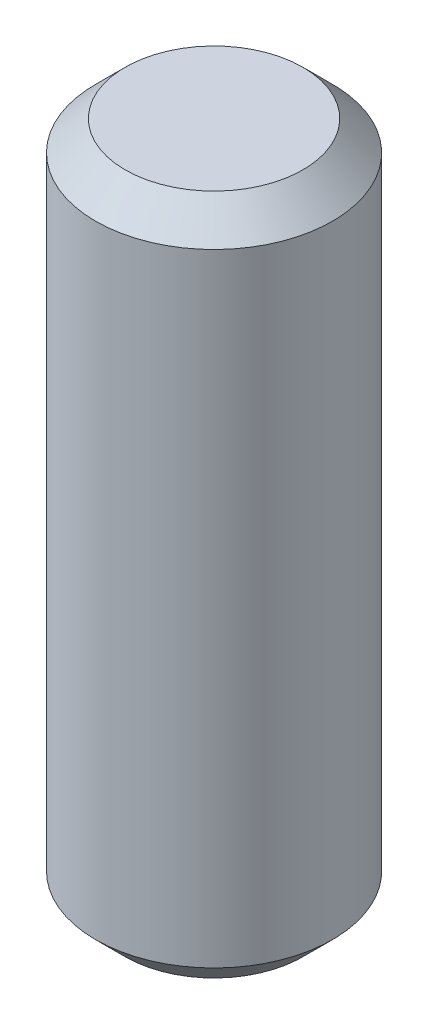
ISO-10303-21;
HEADER;
FILE_DESCRIPTION(('STEP AP214'),'2;1');
FILE_NAME('part.step','',(''),(''),'','','');
FILE_SCHEMA(('AUTOMOTIVE_DESIGN { 1 0 10303 214 1 1 1 1 }'));
ENDSEC;
DATA;
#1=APPLICATION_CONTEXT('core data for automotive mechanical design processes');
#2=APPLICATION_PROTOCOL_DEFINITION('international standard','automotive_design',2000,#1);
#3=PRODUCT_CONTEXT('',#1,'mechanical');
#4=PRODUCT('Part','Part','',(#3));
#5=PRODUCT_RELATED_PRODUCT_CATEGORY('part','',(#4));
#6=PRODUCT_DEFINITION_FORMATION('','',#4);
#7=PRODUCT_DEFINITION_CONTEXT('part definition',#1,'design');
#8=PRODUCT_DEFINITION('design','',#6,#7);
#9=PRODUCT_DEFINITION_SHAPE('','',#8);
#10=(LENGTH_UNIT() NAMED_UNIT(*) SI_UNIT(.MILLI.,.METRE.));
#11=(NAMED_UNIT(*) PLANE_ANGLE_UNIT() SI_UNIT($,.RADIAN.));
#12=(NAMED_UNIT(*) SI_UNIT($,.STERADIAN.) SOLID_ANGLE_UNIT());
#13=UNCERTAINTY_MEASURE_WITH_UNIT(LENGTH_MEASURE(1.E-05),#10,'distance_accuracy_value','');
#14=(GEOMETRIC_REPRESENTATION_CONTEXT(3) GLOBAL_UNCERTAINTY_ASSIGNED_CONTEXT((#13)) GLOBAL_UNIT_ASSIGNED_CONTEXT((#10,
#11,#12)) REPRESENTATION_CONTEXT('',''));
#15=CARTESIAN_POINT('',(0.,0.,0.));
#16=DIRECTION('',(0.,0.,1.));
#17=DIRECTION('',(1.,0.,0.));
#18=AXIS2_PLACEMENT_3D('',#15,#16,#17);
#19=CARTESIAN_POINT('',(0.,11.5,0.));
#20=DIRECTION('',(0.,-1.,0.));
#21=DIRECTION('',(0.,0.,-1.));
#22=AXIS2_PLACEMENT_3D('',#19,#20,#21);
#23=CYLINDRICAL_SURFACE('',#22,2.);
#24=CARTESIAN_POINT('',(0.,0.500000000000002,0.));
#25=DIRECTION('',(0.,1.,0.));
#26=DIRECTION('',(0.,0.,1.));
#27=AXIS2_PLACEMENT_3D('',#24,#25,#26);
#28=CIRCLE('',#27,2.);
#29=CARTESIAN_POINT('',(0.,0.500000000000002,2.));
#30=VERTEX_POINT('',#29);
#31=EDGE_CURVE('E47',#30,#30,#28,.T.);
#32=ORIENTED_EDGE('',*,*,#31,.T.);
#33=EDGE_LOOP('',(#32));
#34=FACE_BOUND('',#33,.T.);
#35=CARTESIAN_POINT('',(0.,11.,0.));
#36=DIRECTION('',(0.,1.,0.));
#37=DIRECTION('',(0.,0.,1.));
#38=AXIS2_PLACEMENT_3D('',#35,#36,#37);
#39=CIRCLE('',#38,2.);
#40=CARTESIAN_POINT('',(0.,11.,2.));
#41=VERTEX_POINT('',#40);
#42=EDGE_CURVE('E52',#41,#41,#39,.F.);
#43=ORIENTED_EDGE('',*,*,#42,.T.);
#44=EDGE_LOOP('',(#43));
#45=FACE_BOUND('',#44,.T.);
#46=ADVANCED_FACE('F41',(#34,#45),#23,.T.);
#47=CARTESIAN_POINT('',(0.,11.5,0.));
#48=DIRECTION('',(0.,1.,0.));
#49=DIRECTION('',(0.,0.,1.));
#50=AXIS2_PLACEMENT_3D('',#47,#48,#49);
#51=PLANE('',#50);
#52=CARTESIAN_POINT('',(0.,11.5,0.));
#53=DIRECTION('',(0.,1.,0.));
#54=DIRECTION('',(0.,0.,1.));
#55=AXIS2_PLACEMENT_3D('',#52,#53,#54);
#56=CIRCLE('',#55,1.5);
#57=CARTESIAN_POINT('',(0.,11.5,1.5));
#58=VERTEX_POINT('',#57);
#59=EDGE_CURVE('E60',#58,#58,#56,.T.);
#60=ORIENTED_EDGE('',*,*,#59,.T.);
#61=EDGE_LOOP('',(#60));
#62=FACE_BOUND('',#61,.T.);
#63=ADVANCED_FACE('F62',(#62),#51,.T.);
#64=CARTESIAN_POINT('',(0.,0.,0.));
#65=DIRECTION('',(0.,1.,0.));
#66=DIRECTION('',(0.,0.,1.));
#67=AXIS2_PLACEMENT_3D('',#64,#65,#66);
#68=PLANE('',#67);
#69=CARTESIAN_POINT('',(0.,0.,0.));
#70=DIRECTION('',(0.,1.,0.));
#71=DIRECTION('',(0.,0.,1.));
#72=AXIS2_PLACEMENT_3D('',#69,#70,#71);
#73=CIRCLE('',#72,1.5);
#74=CARTESIAN_POINT('',(0.,0.,1.5));
#75=VERTEX_POINT('',#74);
#76=EDGE_CURVE('E10',#75,#75,#73,.F.);
#77=ORIENTED_EDGE('',*,*,#76,.T.);
#78=EDGE_LOOP('',(#77));
#79=FACE_BOUND('',#78,.T.);
#80=ADVANCED_FACE('F70',(#79),#68,.F.);
#81=CARTESIAN_POINT('',(0.,11.5,0.));
#82=DIRECTION('',(0.,-1.,0.));
#83=DIRECTION('',(0.,0.,-1.));
#84=AXIS2_PLACEMENT_3D('',#81,#82,#83);
#85=CONICAL_SURFACE('',#84,1.5,0.785398163397447);
#86=ORIENTED_EDGE('',*,*,#42,.F.);
#87=EDGE_LOOP('',(#86));
#88=FACE_BOUND('',#87,.T.);
#89=ORIENTED_EDGE('',*,*,#59,.F.);
#90=EDGE_LOOP('',(#89));
#91=FACE_BOUND('',#90,.T.);
#92=ADVANCED_FACE('F61',(#88,#91),#85,.T.);
#93=CARTESIAN_POINT('',(0.,0.500000000000002,0.));
#94=DIRECTION('',(0.,1.,0.));
#95=DIRECTION('',(0.,0.,1.));
#96=AXIS2_PLACEMENT_3D('',#93,#94,#95);
#97=CONICAL_SURFACE('',#96,2.,0.78539816339745);
#98=ORIENTED_EDGE('',*,*,#76,.F.);
#99=EDGE_LOOP('',(#98));
#100=FACE_BOUND('',#99,.T.);
#101=ORIENTED_EDGE('',*,*,#31,.F.);
#102=EDGE_LOOP('',(#101));
#103=FACE_BOUND('',#102,.T.);
#104=ADVANCED_FACE('F42',(#100,#103),#97,.T.);
#105=CLOSED_SHELL('',(#46,#63,#80,#92,#104));
#106=MANIFOLD_SOLID_BREP('B2',#105);
#107=ADVANCED_BREP_SHAPE_REPRESENTATION('',(#18,#106),#14);
#108=SHAPE_DEFINITION_REPRESENTATION(#9,#107);
ENDSEC;
END-ISO-10303-21;
